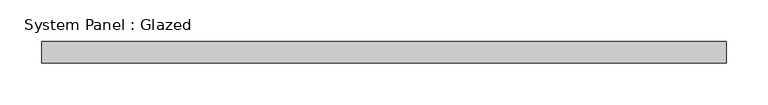
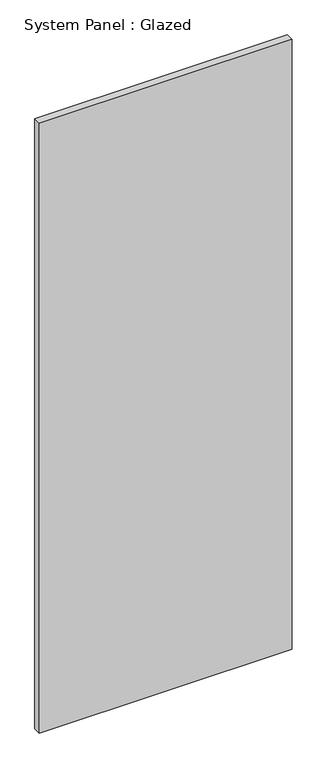
"""IFC4 building model written with IfcOpenShell, lengths in millimetres: plate geometry, System Panel : Glazed."""

from ifc_helpers import new_model, si_unit, origin, origin_with_axes, place, context, project, spatial, polyline, outline, extrude, source, transform, mapped, element, save


def system_panel_glazed_ef5431d1(model_context):
    return source(origin(), model_context, "Body", "SweptSolid", [
        extrude(outline(polyline([(409.575, 19.05), (-409.575, 19.05), (-409.575, 44.45), (409.575, 44.45), (409.575, 19.05)])), origin_with_axes(), (0.0, 0.0, 1.0), 2087.7649104),
    ])


if __name__ == "__main__":
    model = new_model("IFC4")
    model_context = context("Model", 3, world=origin())
    ifc_project = project(units=[si_unit("LENGTHUNIT", "METRE", prefix="MILLI")], contexts=[model_context])
    site = spatial("IfcSite", under=ifc_project)
    building = spatial("IfcBuilding", under=site)
    placement = place(None, origin())
    system_panel_glazed_shape = system_panel_glazed_ef5431d1(model_context)
    element("IfcPlate", 1, ObjectType="System Panel : Glazed", at=placement, inside=building, context=model_context, shape_type="MappedRepresentation", body=[
        mapped(system_panel_glazed_shape, transform((0.0, 0.0, 0.0), x_axis=(1.0, 0.0, 0.0), y_axis=(0.0, 1.0, 0.0), z_axis=(0.0, 0.0, 1.0))),
    ])
    save(model, "model.ifc")

# Revit data of these elements
# Type "System Panel : Glazed"
#   Construction Type Id = "GSP4R"
#   Analytic Construction = "1/8 in Pilkington single glazing"
#   Visual Light Transmittance = 0.9
#   Solar Heat Gain Coefficient = 0.86
#   Heat Transfer Coefficient (U) = 1.18115 BTU/(h·ft²·°F)
#   Define Thermal Properties by = 1
# Element 1 (IfcPlate, "System Panel : Glazed")
#   Materials on its faces: "Glass"
# Materials
#   "Glass": class "Glass", colour RGB 0 128 192, transparency 0.75, Description = "Soda Lime Glass", Cost = 0
